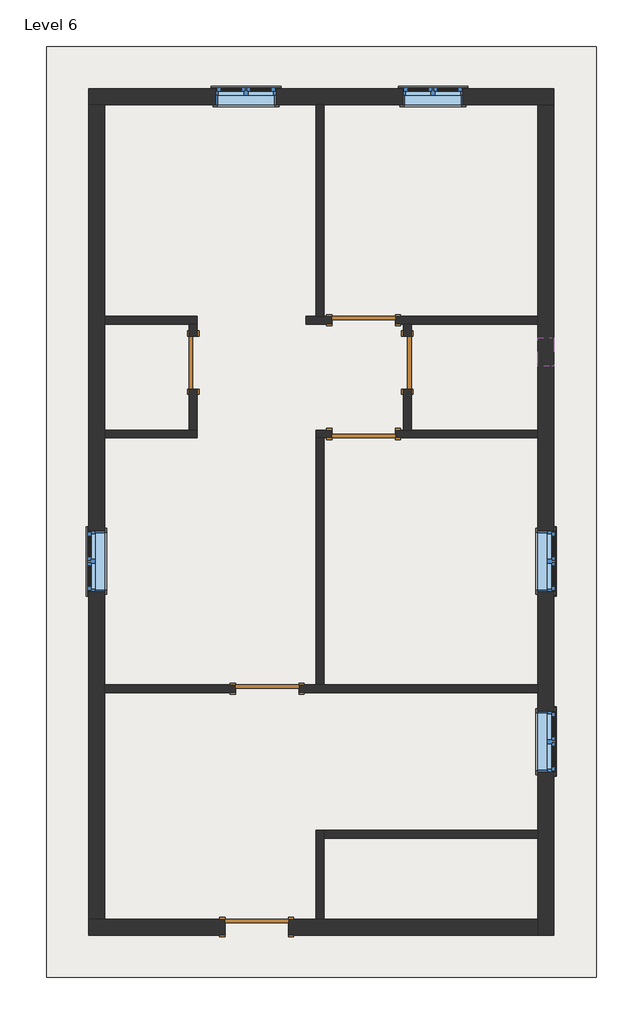
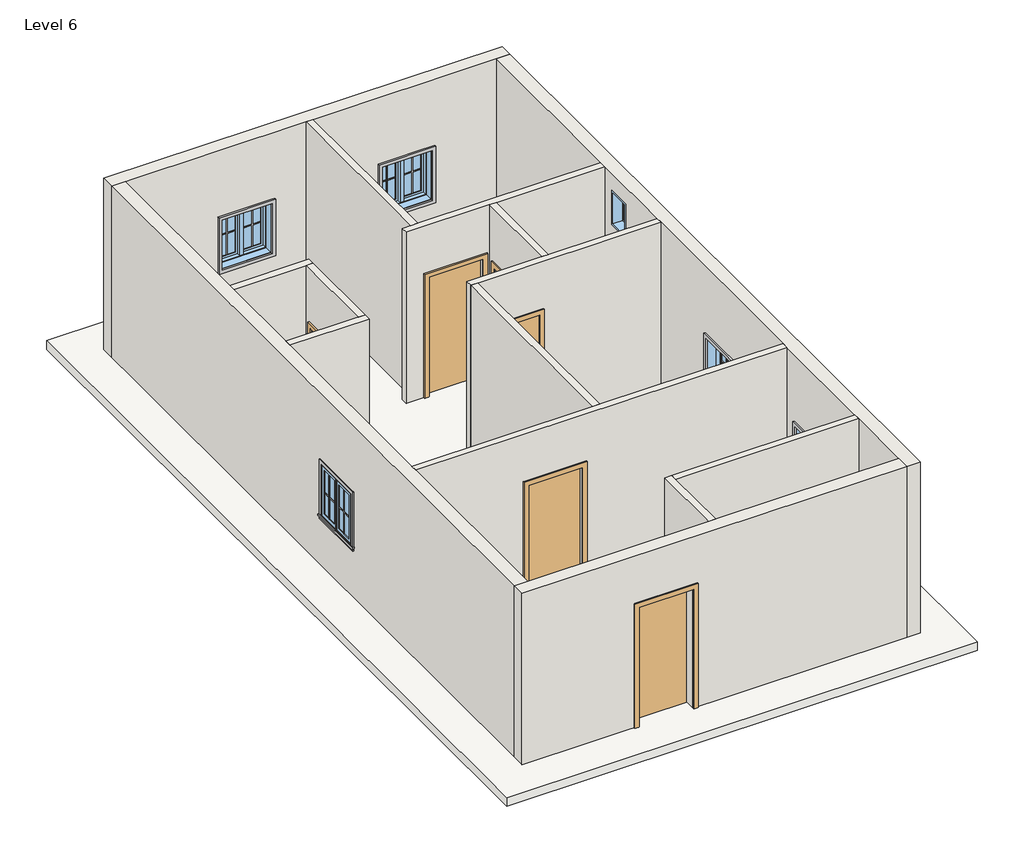
# One storey, incomplete: 20 proxies, 15 walls, 6 doors, 6 windows, 1 roof.
"""IFC4 building model written with IfcOpenShell, lengths in millimetres."""

from ifc_helpers import new_model, si_unit, frame, origin, place, context, project, spatial, polyline, outline, extrude, faceted_brep, transform, mapped, element, save
from components import muntin_pattern_2x2_muntin_pattern_2x2_b3fe6957, muntin_pattern_2x2_muntin_pattern_2x2_3e0ecaf2, trim_window_exterior_flat_with_sill_41619996, trim_window_interior_flat_picture_frame_51c85655, door_f2b275c1, door_d8f5dbb5, door_305aa2a5, door_e5f9f3c4, door_a90ba1ad, window_aa618e30, window_339605e1

model = new_model("IFC4")

# Units and contexts
model_context = context("Model", 3, world=origin())
ifc_project = project(units=[si_unit("LENGTHUNIT", "METRE", prefix="MILLI")], contexts=[model_context])

# Site, building, storey
site = spatial("IfcSite", under=ifc_project)
building = spatial("IfcBuilding", under=site)
storey = spatial("IfcBuildingStorey", under=building, Name="Level 6", Elevation=12801.6)

# Proxies
placement = place(None, origin())
muntin_pattern_2x2_muntin_pattern_2x2_shape = muntin_pattern_2x2_muntin_pattern_2x2_b3fe6957(model_context)
element("IfcBuildingElementProxy", 1, Name="Muntin Pattern_2x2 : Muntin Pattern_2x2", ObjectType="Muntin Pattern_2x2 : Muntin Pattern_2x2", at=placement, inside=storey, context=model_context, shape_type="MappedRepresentation", body=[
    mapped(muntin_pattern_2x2_muntin_pattern_2x2_shape, transform((-2560.703247, 6624.6685985, 13785.85), x_axis=(1.0, 0.0, 0.0), y_axis=(0.0, 1.0, 0.0), z_axis=(0.0, 0.0, 1.0))),
])
element("IfcBuildingElementProxy", 2, Name="Muntin Pattern_2x2 : Muntin Pattern_2x2", ObjectType="Muntin Pattern_2x2 : Muntin Pattern_2x2", at=placement, inside=storey, context=model_context, shape_type="MappedRepresentation", body=[
    mapped(muntin_pattern_2x2_muntin_pattern_2x2_shape, transform((134.871753, 6624.6685985, 13785.85), x_axis=(1.0, 0.0, 0.0), y_axis=(0.0, 1.0, 0.0), z_axis=(0.0, 0.0, 1.0))),
])
element("IfcBuildingElementProxy", 3, Name="Muntin Pattern_2x2 : Muntin Pattern_2x2", ObjectType="Muntin Pattern_2x2 : Muntin Pattern_2x2", at=placement, inside=storey, context=model_context, shape_type="MappedRepresentation", body=[
    mapped(muntin_pattern_2x2_muntin_pattern_2x2_shape, transform((2082.734253, 41.3060985, 13785.85), x_axis=(0.0, -1.0, 0.0), y_axis=(1.0, 0.0, 0.0), z_axis=(0.0, 0.0, 1.0))),
])
element("IfcBuildingElementProxy", 4, Name="Muntin Pattern_2x2 : Muntin Pattern_2x2", ObjectType="Muntin Pattern_2x2 : Muntin Pattern_2x2", at=placement, inside=storey, context=model_context, shape_type="MappedRepresentation", body=[
    mapped(muntin_pattern_2x2_muntin_pattern_2x2_shape, transform((-4603.815747, -387.3189015, 13785.85), x_axis=(0.0, 1.0, 0.0), y_axis=(-1.0, 0.0, 0.0), z_axis=(0.0, 0.0, 1.0))),
])
element("IfcBuildingElementProxy", 5, Name="Muntin Pattern_2x2 : Muntin Pattern_2x2", ObjectType="Muntin Pattern_2x2 : Muntin Pattern_2x2", at=placement, inside=storey, context=model_context, shape_type="MappedRepresentation", body=[
    mapped(muntin_pattern_2x2_muntin_pattern_2x2_shape, transform((2082.734253, -2555.8439015, 13785.85), x_axis=(0.0, -1.0, 0.0), y_axis=(1.0, 0.0, 0.0), z_axis=(0.0, 0.0, 1.0))),
])
muntin_pattern_2x2_muntin_pattern_2x2_2_shape = muntin_pattern_2x2_muntin_pattern_2x2_3e0ecaf2(model_context)
element("IfcBuildingElementProxy", 6, Name="Muntin Pattern_2x2 : Muntin Pattern_2x2", ObjectType="Muntin Pattern_2x2 : Muntin Pattern_2x2", at=placement, inside=storey, context=model_context, shape_type="MappedRepresentation", body=[
    mapped(muntin_pattern_2x2_muntin_pattern_2x2_2_shape, transform((-2132.078247, 6624.6685985, 13785.85), x_axis=(-1.0, 0.0, 0.0), y_axis=(0.0, -1.0, 0.0), z_axis=(0.0, 0.0, 1.0))),
])
element("IfcBuildingElementProxy", 7, Name="Muntin Pattern_2x2 : Muntin Pattern_2x2", ObjectType="Muntin Pattern_2x2 : Muntin Pattern_2x2", at=placement, inside=storey, context=model_context, shape_type="MappedRepresentation", body=[
    mapped(muntin_pattern_2x2_muntin_pattern_2x2_2_shape, transform((563.496753, 6624.6685985, 13785.85), x_axis=(-1.0, 0.0, 0.0), y_axis=(0.0, -1.0, 0.0), z_axis=(0.0, 0.0, 1.0))),
])
element("IfcBuildingElementProxy", 8, Name="Muntin Pattern_2x2 : Muntin Pattern_2x2", ObjectType="Muntin Pattern_2x2 : Muntin Pattern_2x2", at=placement, inside=storey, context=model_context, shape_type="MappedRepresentation", body=[
    mapped(muntin_pattern_2x2_muntin_pattern_2x2_2_shape, transform((2082.734253, -387.3189015, 13785.85), x_axis=(0.0, 1.0, 0.0), y_axis=(-1.0, 0.0, 0.0), z_axis=(0.0, 0.0, 1.0))),
])
element("IfcBuildingElementProxy", 9, Name="Muntin Pattern_2x2 : Muntin Pattern_2x2", ObjectType="Muntin Pattern_2x2 : Muntin Pattern_2x2", at=placement, inside=storey, context=model_context, shape_type="MappedRepresentation", body=[
    mapped(muntin_pattern_2x2_muntin_pattern_2x2_2_shape, transform((-4603.815747, 41.3060985, 13785.85), x_axis=(0.0, -1.0, 0.0), y_axis=(1.0, 0.0, 0.0), z_axis=(0.0, 0.0, 1.0))),
])
element("IfcBuildingElementProxy", 10, Name="Muntin Pattern_2x2 : Muntin Pattern_2x2", ObjectType="Muntin Pattern_2x2 : Muntin Pattern_2x2", at=placement, inside=storey, context=model_context, shape_type="MappedRepresentation", body=[
    mapped(muntin_pattern_2x2_muntin_pattern_2x2_2_shape, transform((2082.734253, -2984.4689015, 13785.85), x_axis=(0.0, 1.0, 0.0), y_axis=(-1.0, 0.0, 0.0), z_axis=(0.0, 0.0, 1.0))),
])
trim_window_exterior_flat_with_sill_shape = trim_window_exterior_flat_with_sill_41619996(model_context)
element("IfcBuildingElementProxy", 11, Name="Trim-Window-Exterior-Flat : with Sill", ObjectType="Trim-Window-Exterior-Flat : with Sill", at=placement, inside=storey, context=model_context, shape_type="MappedRepresentation", body=[
    mapped(trim_window_exterior_flat_with_sill_shape, transform((-2346.390747, 6634.1935985, 14630.4), x_axis=(-1.0, 0.0, 0.0), y_axis=(0.0, 0.0, 1.0), z_axis=(0.0, 1.0, 0.0))),
])
element("IfcBuildingElementProxy", 12, Name="Trim-Window-Exterior-Flat : with Sill", ObjectType="Trim-Window-Exterior-Flat : with Sill", at=placement, inside=storey, context=model_context, shape_type="MappedRepresentation", body=[
    mapped(trim_window_exterior_flat_with_sill_shape, transform((349.184253, 6634.1935985, 14630.4), x_axis=(-1.0, 0.0, 0.0), y_axis=(0.0, 0.0, 1.0), z_axis=(0.0, 1.0, 0.0))),
])
element("IfcBuildingElementProxy", 13, Name="Trim-Window-Exterior-Flat : with Sill", ObjectType="Trim-Window-Exterior-Flat : with Sill", at=placement, inside=storey, context=model_context, shape_type="MappedRepresentation", body=[
    mapped(trim_window_exterior_flat_with_sill_shape, transform((2092.259253, -173.0064015, 14630.4), x_axis=(0.0, 1.0, 0.0), y_axis=(0.0, 0.0, 1.0), z_axis=(1.0, 0.0, 0.0))),
])
element("IfcBuildingElementProxy", 14, Name="Trim-Window-Exterior-Flat : with Sill", ObjectType="Trim-Window-Exterior-Flat : with Sill", at=placement, inside=storey, context=model_context, shape_type="MappedRepresentation", body=[
    mapped(trim_window_exterior_flat_with_sill_shape, transform((-4613.340747, -173.0064015, 14630.4), x_axis=(0.0, -1.0, 0.0), y_axis=(0.0, 0.0, 1.0), z_axis=(-1.0, 0.0, 0.0))),
])
element("IfcBuildingElementProxy", 15, Name="Trim-Window-Exterior-Flat : with Sill", ObjectType="Trim-Window-Exterior-Flat : with Sill", at=placement, inside=storey, context=model_context, shape_type="MappedRepresentation", body=[
    mapped(trim_window_exterior_flat_with_sill_shape, transform((2092.259253, -2770.1564015, 14630.4), x_axis=(0.0, 1.0, 0.0), y_axis=(0.0, 0.0, 1.0), z_axis=(1.0, 0.0, 0.0))),
])
trim_window_interior_flat_picture_frame_shape = trim_window_interior_flat_picture_frame_51c85655(model_context)
element("IfcBuildingElementProxy", 16, Name="Trim-Window-Interior-Flat : Picture Frame", ObjectType="Trim-Window-Interior-Flat : Picture Frame", at=placement, inside=storey, context=model_context, shape_type="MappedRepresentation", body=[
    mapped(trim_window_interior_flat_picture_frame_shape, transform((-2346.390747, 6405.5935985, 14630.4), x_axis=(1.0, 0.0, 0.0), y_axis=(0.0, 0.0, 1.0), z_axis=(0.0, -1.0, 0.0))),
])
element("IfcBuildingElementProxy", 17, Name="Trim-Window-Interior-Flat : Picture Frame", ObjectType="Trim-Window-Interior-Flat : Picture Frame", at=placement, inside=storey, context=model_context, shape_type="MappedRepresentation", body=[
    mapped(trim_window_interior_flat_picture_frame_shape, transform((349.184253, 6405.5935985, 14630.4), x_axis=(1.0, 0.0, 0.0), y_axis=(0.0, 0.0, 1.0), z_axis=(0.0, -1.0, 0.0))),
])
element("IfcBuildingElementProxy", 18, Name="Trim-Window-Interior-Flat : Picture Frame", ObjectType="Trim-Window-Interior-Flat : Picture Frame", at=placement, inside=storey, context=model_context, shape_type="MappedRepresentation", body=[
    mapped(trim_window_interior_flat_picture_frame_shape, transform((1863.659253, -173.0064015, 14630.4), x_axis=(0.0, -1.0, 0.0), y_axis=(0.0, 0.0, 1.0), z_axis=(-1.0, 0.0, 0.0))),
])
element("IfcBuildingElementProxy", 19, Name="Trim-Window-Interior-Flat : Picture Frame", ObjectType="Trim-Window-Interior-Flat : Picture Frame", at=placement, inside=storey, context=model_context, shape_type="MappedRepresentation", body=[
    mapped(trim_window_interior_flat_picture_frame_shape, transform((-4384.740747, -173.0064015, 14630.4), x_axis=(0.0, 1.0, 0.0), y_axis=(0.0, 0.0, 1.0), z_axis=(1.0, 0.0, 0.0))),
])
element("IfcBuildingElementProxy", 20, Name="Trim-Window-Interior-Flat : Picture Frame", ObjectType="Trim-Window-Interior-Flat : Picture Frame", at=placement, inside=storey, context=model_context, shape_type="MappedRepresentation", body=[
    mapped(trim_window_interior_flat_picture_frame_shape, transform((1863.659253, -2770.1564015, 14630.4), x_axis=(0.0, -1.0, 0.0), y_axis=(0.0, 0.0, 1.0), z_axis=(-1.0, 0.0, 0.0))),
])

# Doors
door_shape = door_f2b275c1(model_context)
element("IfcDoor", 21, ObjectType="Single-Flush : 30\" x 80\"", at=placement, inside=storey, context=model_context, shape_type="MappedRepresentation", body=[
    mapped(door_shape, transform((-22.290747, 2690.8435985, 12801.6), x_axis=(0.0, 1.0, 0.0), y_axis=(-1.0, 0.0, 0.0), z_axis=(0.0, 0.0, 1.0))),
])
door_2_shape = door_d8f5dbb5(model_context)
element("IfcDoor", 22, ObjectType="Single-Flush : 30\" x 80\"", at=placement, inside=storey, context=model_context, shape_type="MappedRepresentation", body=[
    mapped(door_2_shape, transform((-3108.390747, 2690.8435985, 12801.6), x_axis=(0.0, 1.0, 0.0), y_axis=(-1.0, 0.0, 0.0), z_axis=(0.0, 0.0, 1.0))),
])
door_3_shape = door_305aa2a5(model_context)
element("IfcDoor", 23, ObjectType="Single-Flush : 36\" x 84\"", at=placement, inside=storey, context=model_context, shape_type="MappedRepresentation", body=[
    mapped(door_3_shape, transform((-650.940747, 3300.4435985, 12801.6), x_axis=(-1.0, 0.0, 0.0), y_axis=(0.0, -1.0, 0.0), z_axis=(0.0, 0.0, 1.0))),
])
door_4_shape = door_e5f9f3c4(model_context)
element("IfcDoor", 24, ObjectType="Single-Flush : 36\" x 84\"", at=placement, inside=storey, context=model_context, shape_type="MappedRepresentation", body=[
    mapped(door_4_shape, transform((-2041.590747, -2008.1564015, 12801.6), x_axis=(1.0, 0.0, 0.0), y_axis=(0.0, 1.0, 0.0), z_axis=(0.0, 0.0, 1.0))),
])
element("IfcDoor", 25, ObjectType="Single-Flush : 36\" x 84\"", at=placement, inside=storey, context=model_context, shape_type="MappedRepresentation", body=[
    mapped(door_4_shape, transform((-650.940747, 1662.1435985, 12801.6), x_axis=(-1.0, 0.0, 0.0), y_axis=(0.0, -1.0, 0.0), z_axis=(0.0, 0.0, 1.0))),
])
door_5_shape = door_a90ba1ad(model_context)
element("IfcDoor", 26, ObjectType="Single-Flush : 36\" x 84\"", at=placement, inside=storey, context=model_context, shape_type="MappedRepresentation", body=[
    mapped(door_5_shape, transform((-2193.990747, -5443.5064015, 12801.6), x_axis=(-1.0, 0.0, 0.0), y_axis=(0.0, -1.0, 0.0), z_axis=(0.0, 0.0, 1.0))),
])

# Roof
element("IfcRoof", 27, ObjectType="Generic - 12\"", at=placement, inside=storey, context=model_context, shape_type="SweptSolid", body=[
    extrude(outline(polyline([(-5222.940747, 7243.7935985), (2701.859253, 7243.7935985), (2701.859253, -6167.4064015), (-5222.940747, -6167.4064015), (-5222.940747, 7243.7935985)])), frame((0.0, 0.0, 12649.2), z_axis=(0.0, 0.0, 1.0), x_axis=(1.0, 0.0, 0.0)), (0.0, 0.0, 1.0), 152.4),
])

# Walls
element("IfcWall", 28, ObjectType="WALL4.5\"", at=placement, inside=storey, context=model_context, shape_type="Brep", body=[
    faceted_brep([(-4384.740747, 3243.2935985, 12801.6), (-3165.540747, 3243.2935985, 12801.6), (-3051.240747, 3243.2935985, 12801.6), (-3051.240747, 3243.2935985, 15849.6), (-3165.540747, 3243.2935985, 15849.6), (-4384.740747, 3243.2935985, 15849.6), (-4384.740747, 3357.5935985, 12801.6), (-4384.740747, 3357.5935985, 15849.6), (-3051.240747, 3357.5935985, 15849.6), (-3051.240747, 3357.5935985, 12801.6)], [[[0, 1, 2, 3, 4, 5]], [[6, 7, 8, 9]], [[2, 1, 0, 6, 9]], [[0, 5, 7, 6]], [[3, 2, 9, 8]], [[5, 4, 3, 8, 7]]]),
])
element("IfcWall", 29, ObjectType="WALL4.5\"", at=placement, inside=storey, context=model_context, shape_type="Brep", body=[
    faceted_brep([(-4384.740747, 1604.9935985, 12801.6), (-3051.240747, 1604.9935985, 12801.6), (-3051.240747, 1604.9935985, 15849.6), (-4384.740747, 1604.9935985, 15849.6), (-4384.740747, 1719.2935985, 12801.6), (-4384.740747, 1719.2935985, 15849.6), (-3165.540747, 1719.2935985, 15849.6), (-3051.240747, 1719.2935985, 15849.6), (-3051.240747, 1719.2935985, 12801.6), (-3165.540747, 1719.2935985, 12801.6)], [[[0, 1, 2, 3]], [[4, 5, 6, 7, 8, 9]], [[1, 0, 4, 9, 8]], [[0, 3, 5, 4]], [[2, 1, 8, 7]], [[3, 2, 7, 6, 5]]]),
])
element("IfcWall", 30, ObjectType="WALL4.5\"", at=placement, inside=storey, context=model_context, shape_type="SweptSolid", body=[
    extrude(outline(polyline([(3243.2935985, 12801.6), (3071.8435985, 12801.6), (3071.8435985, 14833.6), (2309.8435985, 14833.6), (2309.8435985, 12801.6), (1719.2935985, 12801.6), (1719.2935985, 15849.6), (3243.2935985, 15849.6), (3243.2935985, 12801.6)])), frame((-3165.540747, 0.0, 0.0), z_axis=(1.0, 0.0, 0.0), x_axis=(0.0, 1.0, 0.0)), (0.0, 0.0, 1.0), 114.3),
])
element("IfcWall", 31, ObjectType="WALL4.5\"", at=placement, inside=storey, context=model_context, shape_type="SweptSolid", body=[
    extrude(outline(polyline([(-1336.740747, 3357.5935985), (-1336.740747, 6405.5935985), (-1222.440747, 6405.5935985), (-1222.440747, 3357.5935985), (-1336.740747, 3357.5935985)])), frame((0.0, 0.0, 12801.6), z_axis=(0.0, 0.0, 1.0), x_axis=(1.0, 0.0, 0.0)), (0.0, 0.0, 1.0), 3048.0),
])
element("IfcWall", 32, ObjectType="WALL4.5\"", at=placement, inside=storey, context=model_context, shape_type="Brep", body=[
    faceted_brep([(-1481.7019184, 3243.2935985, 12801.6), (-1108.140747, 3243.2935985, 12801.6), (-1108.140747, 3243.2935985, 14935.2), (-193.740747, 3243.2935985, 14935.2), (-193.740747, 3243.2935985, 12801.6), (-79.440747, 3243.2935985, 12801.6), (34.859253, 3243.2935985, 12801.6), (1863.659253, 3243.2935985, 12801.6), (1863.659253, 3243.2935985, 15849.6), (34.859253, 3243.2935985, 15849.6), (-79.440747, 3243.2935985, 15849.6), (-1481.7019184, 3243.2935985, 15849.6), (-1108.140747, 3357.5935985, 14935.2), (-1108.140747, 3357.5935985, 12801.6), (-1222.440747, 3357.5935985, 12801.6), (-1336.740747, 3357.5935985, 12801.6), (-1481.7019184, 3357.5935985, 12801.6), (-1481.7019184, 3357.5935985, 15849.6), (-1336.740747, 3357.5935985, 15849.6), (-1222.440747, 3357.5935985, 15849.6), (1863.659253, 3357.5935985, 15849.6), (1863.659253, 3357.5935985, 12801.6), (-193.740747, 3357.5935985, 12801.6), (-193.740747, 3357.5935985, 14935.2)], [[[0, 1, 2, 3, 4, 5, 6, 7, 8, 9, 10, 11]], [[12, 13, 14, 15, 16, 17, 18, 19, 20, 21, 22, 23]], [[22, 21, 7, 6, 5, 4]], [[16, 15, 14, 13, 1, 0]], [[0, 11, 17, 16]], [[8, 7, 21, 20]], [[2, 1, 13, 12]], [[3, 2, 12, 23]], [[4, 3, 23, 22]], [[11, 10, 9, 8, 20, 19, 18, 17]]]),
])
element("IfcWall", 33, ObjectType="WALL4.5\"", at=placement, inside=storey, context=model_context, shape_type="SweptSolid", body=[
    extrude(outline(polyline([(3243.2935985, 12801.6), (3071.8435985, 12801.6), (3071.8435985, 14833.6), (2309.8435985, 14833.6), (2309.8435985, 12801.6), (1719.2935985, 12801.6), (1719.2935985, 15849.6), (3243.2935985, 15849.6), (3243.2935985, 12801.6)])), frame((-79.440747, 0.0, 0.0), z_axis=(1.0, 0.0, 0.0), x_axis=(0.0, 1.0, 0.0)), (0.0, 0.0, 1.0), 114.3),
])
element("IfcWall", 34, ObjectType="WALL4.5\"", at=placement, inside=storey, context=model_context, shape_type="Brep", body=[
    faceted_brep([(-1108.140747, 1719.2935985, 14935.2), (-1108.140747, 1719.2935985, 12801.6), (-1336.740747, 1719.2935985, 12801.6), (-1336.740747, 1719.2935985, 15849.6), (-79.440747, 1719.2935985, 15849.6), (34.859253, 1719.2935985, 15849.6), (1863.659253, 1719.2935985, 15849.6), (1863.659253, 1719.2935985, 12801.6), (34.859253, 1719.2935985, 12801.6), (-79.440747, 1719.2935985, 12801.6), (-193.740747, 1719.2935985, 12801.6), (-193.740747, 1719.2935985, 14935.2), (-1336.740747, 1604.9935985, 12801.6), (-1222.440747, 1604.9935985, 12801.6), (-1108.140747, 1604.9935985, 12801.6), (-1108.140747, 1604.9935985, 14935.2), (-193.740747, 1604.9935985, 14935.2), (-193.740747, 1604.9935985, 12801.6), (1863.659253, 1604.9935985, 12801.6), (1863.659253, 1604.9935985, 15849.6), (-1222.440747, 1604.9935985, 15849.6), (-1336.740747, 1604.9935985, 15849.6)], [[[0, 1, 2, 3, 4, 5, 6, 7, 8, 9, 10, 11]], [[12, 13, 14, 15, 16, 17, 18, 19, 20, 21]], [[2, 1, 14, 13, 12]], [[10, 9, 8, 7, 18, 17]], [[7, 6, 19, 18]], [[3, 2, 12, 21]], [[15, 14, 1, 0]], [[16, 15, 0, 11]], [[17, 16, 11, 10]], [[6, 5, 4, 3, 21, 20, 19]]]),
])
element("IfcWall", 35, ObjectType="WALL4.5\"", at=placement, inside=storey, context=model_context, shape_type="SweptSolid", body=[
    extrude(outline(polyline([(-1336.740747, -1951.0064015), (-1336.740747, 1604.9935985), (-1222.440747, 1604.9935985), (-1222.440747, -1951.0064015), (-1336.740747, -1951.0064015)])), frame((0.0, 0.0, 12801.6), z_axis=(0.0, 0.0, 1.0), x_axis=(1.0, 0.0, 0.0)), (0.0, 0.0, 1.0), 3048.0),
])
element("IfcWall", 36, ObjectType="WALL4.5\"", at=placement, inside=storey, context=model_context, shape_type="Brep", body=[
    faceted_brep([(-1584.390747, -2065.3064015, 14935.2), (-1584.390747, -2065.3064015, 12801.6), (1863.659253, -2065.3064015, 12801.6), (1863.659253, -2065.3064015, 15849.6), (-4384.740747, -2065.3064015, 15849.6), (-4384.740747, -2065.3064015, 12801.6), (-2498.790747, -2065.3064015, 12801.6), (-2498.790747, -2065.3064015, 14935.2), (1863.659253, -1951.0064015, 12801.6), (-1222.440747, -1951.0064015, 12801.6), (-1336.740747, -1951.0064015, 12801.6), (-1584.390747, -1951.0064015, 12801.6), (-1584.390747, -1951.0064015, 14935.2), (-2498.790747, -1951.0064015, 14935.2), (-2498.790747, -1951.0064015, 12801.6), (-4384.740747, -1951.0064015, 12801.6), (-4384.740747, -1951.0064015, 15849.6), (-1336.740747, -1951.0064015, 15849.6), (-1222.440747, -1951.0064015, 15849.6), (1863.659253, -1951.0064015, 15849.6)], [[[0, 1, 2, 3, 4, 5, 6, 7]], [[8, 9, 10, 11, 12, 13, 14, 15, 16, 17, 18, 19]], [[6, 5, 15, 14]], [[2, 1, 11, 10, 9, 8]], [[3, 2, 8, 19]], [[5, 4, 16, 15]], [[12, 11, 1, 0]], [[13, 12, 0, 7]], [[14, 13, 7, 6]], [[4, 3, 19, 18, 17, 16]]]),
])
element("IfcWall", 37, ObjectType="WALL4.5\"", at=placement, inside=storey, context=model_context, shape_type="Brep", body=[
    faceted_brep([(-1222.440747, -5329.2064015, 12801.6), (-1222.440747, -4160.8064015, 12801.6), (-1222.440747, -4046.5064015, 12801.6), (-1222.440747, -4046.5064015, 15849.6), (-1222.440747, -4160.8064015, 15849.6), (-1222.440747, -5329.2064015, 15849.6), (-1336.740747, -5329.2064015, 12801.6), (-1336.740747, -5329.2064015, 15849.6), (-1336.740747, -4046.5064015, 15849.6), (-1336.740747, -4046.5064015, 12801.6)], [[[0, 1, 2, 3, 4, 5]], [[6, 7, 8, 9]], [[2, 1, 0, 6, 9]], [[0, 5, 7, 6]], [[3, 2, 9, 8]], [[5, 4, 3, 8, 7]]]),
])
element("IfcWall", 38, ObjectType="WALL4.5\"", at=placement, inside=storey, context=model_context, shape_type="SweptSolid", body=[
    extrude(outline(polyline([(1863.659253, -4160.8064015), (-1222.440747, -4160.8064015), (-1222.440747, -4046.5064015), (1863.659253, -4046.5064015), (1863.659253, -4160.8064015)])), frame((0.0, 0.0, 12801.6), z_axis=(0.0, 0.0, 1.0), x_axis=(1.0, 0.0, 0.0)), (0.0, 0.0, 1.0), 3048.0),
])
element("IfcWall", 39, ObjectType="WALL9\"", at=placement, inside=storey, context=model_context, shape_type="Brep", body=[
    faceted_brep([(-4613.340747, 6405.5935985, 12801.6), (-4384.740747, 6405.5935985, 12801.6), (-1336.740747, 6405.5935985, 12801.6), (-1222.440747, 6405.5935985, 12801.6), (1863.659253, 6405.5935985, 12801.6), (2092.259253, 6405.5935985, 12801.6), (2092.259253, 6405.5935985, 15849.6), (1863.659253, 6405.5935985, 15849.6), (-1222.440747, 6405.5935985, 15849.6), (-1336.740747, 6405.5935985, 15849.6), (-4384.740747, 6405.5935985, 15849.6), (-4613.340747, 6405.5935985, 15849.6), (-1914.590747, 6405.5935985, 14630.4), (-1914.590747, 6405.5935985, 13716.0), (-2778.190747, 6405.5935985, 13716.0), (-2778.190747, 6405.5935985, 14630.4), (780.984253, 6405.5935985, 14630.4), (780.984253, 6405.5935985, 13716.0), (-82.615747, 6405.5935985, 13716.0), (-82.615747, 6405.5935985, 14630.4), (-4613.340747, 6634.1935985, 12801.6), (-4613.340747, 6634.1935985, 15849.6), (2092.259253, 6634.1935985, 15849.6), (2092.259253, 6634.1935985, 12801.6), (-1914.590747, 6634.1935985, 14630.4), (-2778.190747, 6634.1935985, 14630.4), (-2778.190747, 6634.1935985, 13716.0), (-1914.590747, 6634.1935985, 13716.0), (780.984253, 6634.1935985, 14630.4), (-82.615747, 6634.1935985, 14630.4), (-82.615747, 6634.1935985, 13716.0), (780.984253, 6634.1935985, 13716.0)], [[[0, 1, 2, 3, 4, 5, 6, 7, 8, 9, 10, 11], [12, 13, 14, 15], [16, 17, 18, 19]], [[20, 21, 22, 23], [24, 25, 26, 27], [28, 29, 30, 31]], [[5, 4, 3, 2, 1, 0, 20, 23]], [[6, 5, 23, 22]], [[0, 11, 21, 20]], [[13, 12, 24, 27]], [[14, 13, 27, 26]], [[15, 14, 26, 25]], [[12, 15, 25, 24]], [[17, 16, 28, 31]], [[18, 17, 31, 30]], [[19, 18, 30, 29]], [[16, 19, 29, 28]], [[11, 10, 9, 8, 7, 6, 22, 21]]]),
])
element("IfcWall", 40, ObjectType="WALL9\"", at=placement, inside=storey, context=model_context, shape_type="Brep", body=[
    faceted_brep([(1863.659253, 6405.5935985, 12801.6), (1863.659253, 3357.5935985, 12801.6), (1863.659253, 3243.2935985, 12801.6), (1863.659253, 1719.2935985, 12801.6), (1863.659253, 1604.9935985, 12801.6), (1863.659253, -1951.0064015, 12801.6), (1863.659253, -2065.3064015, 12801.6), (1863.659253, -4046.5064015, 12801.6), (1863.659253, -4160.8064015, 12801.6), (1863.659253, -5329.2064015, 12801.6), (1863.659253, -5557.8064015, 12801.6), (1863.659253, -5557.8064015, 15849.6), (1863.659253, -5329.2064015, 15849.6), (1863.659253, -4160.8064015, 15849.6), (1863.659253, -4046.5064015, 15849.6), (1863.659253, -2065.3064015, 15849.6), (1863.659253, -1951.0064015, 15849.6), (1863.659253, 1604.9935985, 15849.6), (1863.659253, 1719.2935985, 15849.6), (1863.659253, 3243.2935985, 15849.6), (1863.659253, 3357.5935985, 15849.6), (1863.659253, 6405.5935985, 15849.6), (1863.659253, 2640.0435985, 15544.8), (1863.659253, 2640.0435985, 14935.2), (1863.659253, 3046.4435985, 14935.2), (1863.659253, 3046.4435985, 15544.8), (1863.659253, -604.8064015, 14630.4), (1863.659253, -604.8064015, 13716.0), (1863.659253, 258.7935985, 13716.0), (1863.659253, 258.7935985, 14630.4), (1863.659253, -3201.9564015, 14630.4), (1863.659253, -3201.9564015, 13716.0), (1863.659253, -2338.3564015, 13716.0), (1863.659253, -2338.3564015, 14630.4), (2092.259253, 6405.5935985, 12801.6), (2092.259253, 6405.5935985, 15849.6), (2092.259253, -5557.8064015, 15849.6), (2092.259253, -5557.8064015, 12801.6), (2092.259253, 2640.0435985, 15544.8), (2092.259253, 3046.4435985, 15544.8), (2092.259253, 3046.4435985, 14935.2), (2092.259253, 2640.0435985, 14935.2), (2092.259253, -604.8064015, 14630.4), (2092.259253, 258.7935985, 14630.4), (2092.259253, 258.7935985, 13716.0), (2092.259253, -604.8064015, 13716.0), (2092.259253, -3201.9564015, 14630.4), (2092.259253, -2338.3564015, 14630.4), (2092.259253, -2338.3564015, 13716.0), (2092.259253, -3201.9564015, 13716.0)], [[[0, 1, 2, 3, 4, 5, 6, 7, 8, 9, 10, 11, 12, 13, 14, 15, 16, 17, 18, 19, 20, 21], [22, 23, 24, 25], [26, 27, 28, 29], [30, 31, 32, 33]], [[34, 35, 36, 37], [38, 39, 40, 41], [42, 43, 44, 45], [46, 47, 48, 49]], [[10, 9, 8, 7, 6, 5, 4, 3, 2, 1, 0, 34, 37]], [[0, 21, 35, 34]], [[11, 10, 37, 36]], [[23, 22, 38, 41]], [[24, 23, 41, 40]], [[25, 24, 40, 39]], [[22, 25, 39, 38]], [[27, 26, 42, 45]], [[28, 27, 45, 44]], [[29, 28, 44, 43]], [[26, 29, 43, 42]], [[31, 30, 46, 49]], [[32, 31, 49, 48]], [[33, 32, 48, 47]], [[30, 33, 47, 46]], [[21, 20, 19, 18, 17, 16, 15, 14, 13, 12, 11, 36, 35]]]),
])
element("IfcWall", 41, ObjectType="WALL9\"", at=placement, inside=storey, context=model_context, shape_type="Brep", body=[
    faceted_brep([(-2651.190747, -5329.2064015, 14935.2), (-2651.190747, -5329.2064015, 12801.6), (-4384.740747, -5329.2064015, 12801.6), (-4613.340747, -5329.2064015, 12801.6), (-4613.340747, -5329.2064015, 15849.6), (-4384.740747, -5329.2064015, 15849.6), (-1336.740747, -5329.2064015, 15849.6), (-1222.440747, -5329.2064015, 15849.6), (1863.659253, -5329.2064015, 15849.6), (1863.659253, -5329.2064015, 12801.6), (-1222.440747, -5329.2064015, 12801.6), (-1336.740747, -5329.2064015, 12801.6), (-1736.790747, -5329.2064015, 12801.6), (-1736.790747, -5329.2064015, 14935.2), (-4613.340747, -5557.8064015, 12801.6), (-2651.190747, -5557.8064015, 12801.6), (-2651.190747, -5557.8064015, 14935.2), (-1736.790747, -5557.8064015, 14935.2), (-1736.790747, -5557.8064015, 12801.6), (1863.659253, -5557.8064015, 12801.6), (1863.659253, -5557.8064015, 15849.6), (-4613.340747, -5557.8064015, 15849.6)], [[[0, 1, 2, 3, 4, 5, 6, 7, 8, 9, 10, 11, 12, 13]], [[14, 15, 16, 17, 18, 19, 20, 21]], [[3, 2, 1, 15, 14]], [[12, 11, 10, 9, 19, 18]], [[9, 8, 20, 19]], [[4, 3, 14, 21]], [[16, 15, 1, 0]], [[17, 16, 0, 13]], [[18, 17, 13, 12]], [[8, 7, 6, 5, 4, 21, 20]]]),
])
element("IfcWall", 42, ObjectType="WALL9\"", at=placement, inside=storey, context=model_context, shape_type="Brep", body=[
    faceted_brep([(-4384.740747, -5329.2064015, 12801.6), (-4384.740747, -2065.3064015, 12801.6), (-4384.740747, -1951.0064015, 12801.6), (-4384.740747, 1604.9935985, 12801.6), (-4384.740747, 1719.2935985, 12801.6), (-4384.740747, 3243.2935985, 12801.6), (-4384.740747, 3357.5935985, 12801.6), (-4384.740747, 6405.5935985, 12801.6), (-4384.740747, 6405.5935985, 15849.6), (-4384.740747, 3357.5935985, 15849.6), (-4384.740747, 3243.2935985, 15849.6), (-4384.740747, 1719.2935985, 15849.6), (-4384.740747, 1604.9935985, 15849.6), (-4384.740747, -1951.0064015, 15849.6), (-4384.740747, -2065.3064015, 15849.6), (-4384.740747, -5329.2064015, 15849.6), (-4384.740747, 258.7935985, 14630.4), (-4384.740747, 258.7935985, 13716.0), (-4384.740747, -604.8064015, 13716.0), (-4384.740747, -604.8064015, 14630.4), (-4613.340747, -5329.2064015, 12801.6), (-4613.340747, -5329.2064015, 15849.6), (-4613.340747, 6405.5935985, 15849.6), (-4613.340747, 6405.5935985, 12801.6), (-4613.340747, 258.7935985, 14630.4), (-4613.340747, -604.8064015, 14630.4), (-4613.340747, -604.8064015, 13716.0), (-4613.340747, 258.7935985, 13716.0)], [[[0, 1, 2, 3, 4, 5, 6, 7, 8, 9, 10, 11, 12, 13, 14, 15], [16, 17, 18, 19]], [[20, 21, 22, 23], [24, 25, 26, 27]], [[7, 6, 5, 4, 3, 2, 1, 0, 20, 23]], [[8, 7, 23, 22]], [[0, 15, 21, 20]], [[17, 16, 24, 27]], [[18, 17, 27, 26]], [[19, 18, 26, 25]], [[16, 19, 25, 24]], [[15, 14, 13, 12, 11, 10, 9, 8, 22, 21]]]),
])

# Windows
window_shape = window_aa618e30(model_context)
element("IfcWindow", 43, ObjectType="Fixed : 16\" x 24\"", at=placement, inside=storey, context=model_context, shape_type="MappedRepresentation", body=[
    mapped(window_shape, transform((1977.959253, 2805.1435985, 14020.8), x_axis=(0.0, -1.0, 0.0), y_axis=(1.0, 0.0, 0.0), z_axis=(0.0, 0.0, 1.0))),
])
window_2_shape = window_339605e1(model_context)
element("IfcWindow", 44, ObjectType="Window-Casement-Double : 34\" x 36\"", at=placement, inside=storey, context=model_context, shape_type="MappedRepresentation", body=[
    mapped(window_2_shape, transform((-2346.390747, 6519.8935985, 12801.6), x_axis=(1.0, 0.0, 0.0), y_axis=(0.0, 1.0, 0.0), z_axis=(0.0, 0.0, 1.0))),
])
element("IfcWindow", 45, ObjectType="Window-Casement-Double : 34\" x 36\"", at=placement, inside=storey, context=model_context, shape_type="MappedRepresentation", body=[
    mapped(window_2_shape, transform((349.184253, 6519.8935985, 12801.6), x_axis=(1.0, 0.0, 0.0), y_axis=(0.0, 1.0, 0.0), z_axis=(0.0, 0.0, 1.0))),
])
element("IfcWindow", 46, ObjectType="Window-Casement-Double : 34\" x 36\"", at=placement, inside=storey, context=model_context, shape_type="MappedRepresentation", body=[
    mapped(window_2_shape, transform((1977.959253, -173.0064015, 12801.6), x_axis=(0.0, -1.0, 0.0), y_axis=(1.0, 0.0, 0.0), z_axis=(0.0, 0.0, 1.0))),
])
element("IfcWindow", 47, ObjectType="Window-Casement-Double : 34\" x 36\"", at=placement, inside=storey, context=model_context, shape_type="MappedRepresentation", body=[
    mapped(window_2_shape, transform((-4499.040747, -173.0064015, 12801.6), x_axis=(0.0, 1.0, 0.0), y_axis=(-1.0, 0.0, 0.0), z_axis=(0.0, 0.0, 1.0))),
])
element("IfcWindow", 48, ObjectType="Window-Casement-Double : 34\" x 36\"", at=placement, inside=storey, context=model_context, shape_type="MappedRepresentation", body=[
    mapped(window_2_shape, transform((1977.959253, -2770.1564015, 12801.6), x_axis=(0.0, -1.0, 0.0), y_axis=(1.0, 0.0, 0.0), z_axis=(0.0, 0.0, 1.0))),
])

save(model, "model.ifc")

# Revit data of these elements
# Type "Muntin Pattern_2x2 : Muntin Pattern_2x2"
#   Width [instance default] = 4' - 0"
#   Thickness = 0' - 0 1/2"
#   Height [instance default] = 4' - 0"
#   Distance = 0' - 0 3/4"
#   Interior Material [instance default] = none
#   Exterior Material [instance default] = none
#   Default Elevation = 0
# Type "Trim-Window-Exterior-Flat : with Sill"
#   Trim Width = 0' - 2 1/4"
#   Trim Thickness_Picture Frame = 0' - 1 1/4"
#   Trim Thickness_with Sill = 0' - 0 3/4"
#   Sill Thickness = 0' - 1 1/4"
#   Opening Width [instance default] = 2' - 0"
#   Opening Height [instance default] = 3' - 0"
#   Default Elevation = 4' - 0"
#   Sill = yes
#   Picture Frame = no
#   Trim Material [instance default] = none
# Type "Trim-Window-Interior-Flat : Picture Frame"
#   Trim Thickness_Picture Frame = 0' - 1 1/4"
#   Trim Width = 0' - 2 1/4"
#   Trim Thickness_with Sill = 0' - 0 3/4"
#   Sill Thickness = 0' - 1 1/4"
#   Opening Width [instance default] = 2' - 0"
#   Opening Height [instance default] = 3' - 0"
#   Default Elevation = 4' - 0"
#   Sill = no
#   Picture Frame = yes
#   Trim Material [instance default] = none
# Type "Single-Flush : 30\" x 80\""
#   Type Mark = "5"
#   Construction Type Id = "MDOOR"
#   Assembly Code = "C1020"
#   Analytic Construction = "Metal"
#   Thickness = 0' - 2"
#   Heat Transfer Coefficient (U) = 0.651978 BTU/(h·ft²·°F)
#   Height = 6' - 8"
#   Trim Projection Ext = 0' - 1"
#   Trim Projection Int = 0' - 1"
#   Trim Width = 0' - 3"
#   Width = 2' - 6"
#   Define Thermal Properties by = 1
#   Define Thermal Properties by = 1
#   Door Material = Door - Panel
#   Frame Material = Door - Frame
#   Visual Light Transmittance = 0
#   Solar Heat Gain Coefficient = 0
#   Function = (empty or 0)
#   Wall Closure = (empty or 0)
# Type "Single-Flush : 36\" x 84\""
#   Type Mark = "1"
#   Construction Type Id = "MDOOR"
#   Assembly Code = "C1020"
#   Analytic Construction = "Metal"
#   Thickness = 0' - 2"
#   Heat Transfer Coefficient (U) = 0.651978 BTU/(h·ft²·°F)
#   Height = 7' - 0"
#   Trim Projection Ext = 0' - 1"
#   Trim Projection Int = 0' - 1"
#   Trim Width = 0' - 3"
#   Width = 3' - 0"
#   Define Thermal Properties by = 1
#   Define Thermal Properties by = 1
#   Door Material = Door - Panel
#   Frame Material = Door - Frame
#   Visual Light Transmittance = 0
#   Solar Heat Gain Coefficient = 0
#   Function = (empty or 0)
#   Wall Closure = (empty or 0)
# Type "Generic - 12\""
#   Assembly Code = "B1020"
#   Layers, outside or top first: 0' - 6" no material (function 1)
# Type "WALL4.5\""
#   Assembly Code = "B2010"
#   Layers, outside or top first: 0' - 4 1/2" no material (function 1)
# Type "WALL9\""
#   Assembly Code = "B2010"
#   Layers, outside or top first: 0' - 9" no material (function 1)
# Type "Fixed : 16\" x 24\""
#   Type Mark = "4"
#   Construction Type Id = "GSP4R"
#   Assembly Code = "B2020100"
#   Analytic Construction = "1/8 in Pilkington single glazing"
#   Visual Light Transmittance = 0.9
#   Solar Heat Gain Coefficient = 0.78
#   Heat Transfer Coefficient (U) = 0.6496 BTU/(h·ft²·°F)
#   Height = 2' - 0"
#   Default Sill Height = 3' - 0"
#   Width = 1' - 4"
#   Window Inset = 0' - 0 3/4"
#   Define Thermal Properties by = 1
#   Define Thermal Properties by = 1
#   Glass Pane Material = Glass
#   Sash Material = Sash
#   Wall Closure = (empty or 0)
# Type "Window-Casement-Double : 34\" x 36\""
#   Type Mark = "14"
#   Fire Rating = "0.5h"
#   Assembly Code = "B2020100"
#   Analytic Construction = "Double glazing - domestic"
#   Frame Extension [instance default] = 0' - 0 1/4"
#   Window Inset [instance default] = 0' - 0"
#   Wall Thickness [instance default] = 0' - 6"
#   Interior Wall Closure [instance default] = 0' - 2 1/4"
#   Half Width = 1' - 5"
#   Visual Light Transmittance = 0.81
#   Thermal Resistance (R) = 1.8146 (h·ft²·°F)/BTU
#   Solar Heat Gain Coefficient = 0.76
#   Rough Width = 2' - 10 1/2"
#   Rough Height = 3' - 0 1/2"
#   Height = 3' - 0"
#   Heat Transfer Coefficient (U) = 0.5511 BTU/(h·ft²·°F)
#   Exterior Wall Closure [instance default] = 0' - 1 1/4"
#   Extension Jamb [instance default] = 0' - 2 1/4"
#   Default Sill Height = 3' - 0"
#   Width = 2' - 10"
#   Define Thermal Properties by = 0
#   Muntin Visibility = yes
#   Interior Trim Visibility [instance default] = yes
#   Exterior Trim Visibility [instance default] = yes
#   Extension Jamb Visibility [instance default] = yes
#   Interior Trim Material = Wood - Stained
#   Muntin Pattern = Muntin Pattern_2x2 : Muntin Pattern_2x2
#   Interior Trim = Trim-Window-Interior-Flat : Picture Frame
#   Interior Frame Material = Wood - Stained
#   Glass Panel Material = Glass
#   Exterior Trim Material = Clad - White
#   Exterior Trim = Trim-Window-Exterior-Flat : with Sill
#   Exterior Frame Material = Clad - White
#   Wall Closure = (empty or 0)
# Elements 1, 2, 3, 4, 5, 6, 7, 8, 9, 10 (IfcBuildingElementProxy, "Muntin Pattern_2x2 : Muntin Pattern_2x2")
#   Width = 0' - 11 5/8"
#   Height = 2' - 6 1/2"
#   Interior Material = Wood - Stained
#   Exterior Material = Clad - White
#   Phase Created = New Construction
#   Materials on its faces: "Clad - White", "Wood - Stained"
# Elements 11, 12, 13, 14, 15 (IfcBuildingElementProxy, "Trim-Window-Exterior-Flat : with Sill")
#   Opening Width = 2' - 10"
#   Opening Height = 3' - 0"
#   Trim Material = Clad - White
#   Phase Created = New Construction
#   Materials on its faces: "Clad - White"
# Elements 16, 17, 18, 19, 20 (IfcBuildingElementProxy, "Trim-Window-Interior-Flat : Picture Frame")
#   Opening Width = 2' - 10"
#   Opening Height = 3' - 0"
#   Trim Material = Wood - Stained
#   Phase Created = New Construction
#   Materials on its faces: "Wood - Stained"
# Elements 21, 22 (IfcDoor, "Single-Flush : 30\" x 80\"")
#   Phase Created = New Construction
#   Materials on its faces: "Door - Frame", "Door - Panel"
# Elements 23, 24, 25, 26 (IfcDoor, "Single-Flush : 36\" x 84\"")
#   Phase Created = New Construction
#   Materials on its faces: "Door - Frame", "Door - Panel"
# Element 27 (IfcRoof, "Generic - 12\"")
#   built-in parameter 1001705 = 42 (stored number, unit not read)
#   built-in parameter 1001701 = -0.5 (stored number, unit not read)
#   built-in parameter 1001710 = 33615
#   Phase Created = New Construction
#   Materials on its faces: "Default Roof", "Door - Panel"
# Elements 28, 29, 30, 31, 32, 33, 34, 35, 36, 37, 38 (IfcWall, "WALL4.5\"")
#   Top Offset = 0' - 0"
#   Base Offset = 0' - 0"
#   Unconnected Height = 10' - 0"
#   wall height = 10' - 0"
#   Phase Created = New Construction
#   Base Constraint = Level 6
#   Materials on its faces: "Default Wall"
# Elements 39, 40, 41, 42 (IfcWall, "WALL9\"")
#   Top Offset = 0' - 0"
#   Base Offset = 0' - 0"
#   Unconnected Height = 10' - 0"
#   wall height = 10' - 0"
#   Phase Created = New Construction
#   Base Constraint = Level 6
#   Materials on its faces: "Default Wall", "Door - Panel"
# Element 43 (IfcWindow, "Fixed : 16\" x 24\"")
#   Mark = "25"
#   Phase Created = New Construction
#   Materials on its faces: "Sash", "Glass"
# Element 44 (IfcWindow, "Window-Casement-Double : 34\" x 36\"")
#   Mark = "26"
#   Window Inset = 0' - 0"
#   Interior Wall Closure = 0' - 2 1/4"
#   Frame Extension = 0' - 0 1/4"
#   Exterior Wall Closure = 0' - 1 1/4"
#   Interior Trim Visibility = yes
#   Exterior Trim Visibility = yes
#   Phase Created = New Construction
#   Materials on its faces: "Wood - Stained", "Glass", "Clad - White"
# Element 45 (IfcWindow, "Window-Casement-Double : 34\" x 36\"")
#   Mark = "27"
#   Window Inset = 0' - 0"
#   Interior Wall Closure = 0' - 2 1/4"
#   Frame Extension = 0' - 0 1/4"
#   Exterior Wall Closure = 0' - 1 1/4"
#   Interior Trim Visibility = yes
#   Exterior Trim Visibility = yes
#   Phase Created = New Construction
#   Materials on its faces: "Wood - Stained", "Glass", "Clad - White"
# Element 46 (IfcWindow, "Window-Casement-Double : 34\" x 36\"")
#   Mark = "28"
#   Window Inset = 0' - 0"
#   Interior Wall Closure = 0' - 2 1/4"
#   Frame Extension = 0' - 0 1/4"
#   Exterior Wall Closure = 0' - 1 1/4"
#   Interior Trim Visibility = yes
#   Exterior Trim Visibility = yes
#   Phase Created = New Construction
#   Materials on its faces: "Wood - Stained", "Glass", "Clad - White"
# Element 47 (IfcWindow, "Window-Casement-Double : 34\" x 36\"")
#   Mark = "29"
#   Window Inset = 0' - 0"
#   Interior Wall Closure = 0' - 2 1/4"
#   Frame Extension = 0' - 0 1/4"
#   Exterior Wall Closure = 0' - 1 1/4"
#   Interior Trim Visibility = yes
#   Exterior Trim Visibility = yes
#   Phase Created = New Construction
#   Materials on its faces: "Wood - Stained", "Glass", "Clad - White"
# Element 48 (IfcWindow, "Window-Casement-Double : 34\" x 36\"")
#   Mark = "30"
#   Window Inset = 0' - 0"
#   Interior Wall Closure = 0' - 2 1/4"
#   Frame Extension = 0' - 0 1/4"
#   Exterior Wall Closure = 0' - 1 1/4"
#   Interior Trim Visibility = yes
#   Exterior Trim Visibility = yes
#   Phase Created = New Construction
#   Materials on its faces: "Wood - Stained", "Glass", "Clad - White"
# Materials
#   "Door - Panel": class "Wood", colour RGB 210 159 95, transparency 0, Cost = 0
#   "Door - Frame": colour RGB 118 70 51, transparency 0, Cost = 0
#   "Glass": class "Glass", colour RGB 0 128 192, transparency 0.75, Description = "Soda Lime Glass", Cost = 0
#   "Sash": class "Wood", colour RGB 224 178 126, transparency 0, Cost = 0
#   "Wood - Stained": class "Wood", colour RGB 224 178 126, transparency 0, Cost = 0
#   "Clad - White": class "Wood", colour RGB 242 242 238, transparency 0, Cost = 0
#   "Default Roof": colour RGB 88 101 114, transparency 0, Cost = 0
#   "Default Wall": colour RGB 128 128 128, transparency 0, Cost = 0
